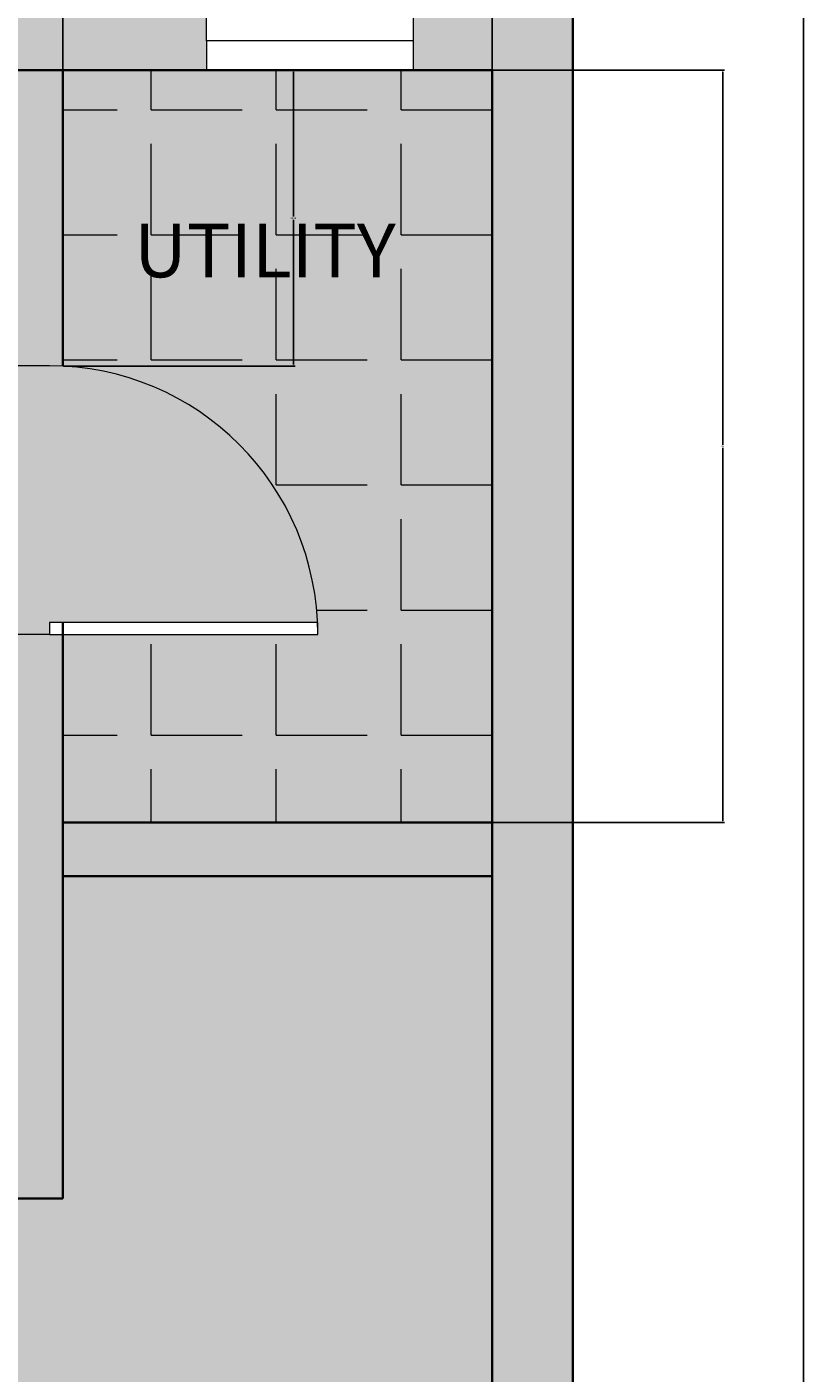
# Model space of a CAD drawing. Units: inches. Extents: x 3024 to 3952, y 1308 to 1863.
# Tile 26 of 29: x 3409 to 3496, y 1633 to 1783. Entities that reach past the tile are written whole.
import ezdxf

# ---------------------------------------------------------------- set-up
doc = ezdxf.new("R2010")
doc.units = ezdxf.units.IN
for name, color, linetype, lineweight in [('A-ANNO-DIMS', 2, 'Continuous', 18), ('A-AREA-IDEN', 7, 'Continuous', 18), ('A-DOOR', 4, 'Continuous', 18), ('A-FLOR-TILE-PATT', 7, 'Continuous', 13), ('A-GLAZ', 4, 'Continuous', 18), ('A-WALL', 7, 'Continuous', 35)]:
    doc.layers.add(name, color=color, linetype=linetype, lineweight=lineweight)
doc.layers.add('A-FLOR-PATT', color=254, linetype='Continuous', lineweight=13, true_color=0xfeeab9)
doc.layers.add('A-WALL-PATT', color=254, linetype='Continuous', lineweight=13, true_color=0xcecce6)
doc.styles.get("Standard").update_dxf_attribs({"font": 'arial.ttf'})
doc.dimstyles.get("Standard").update_dxf_attribs({"dimtxt": 0.18, "dimasz": 0.18, "dimexe": 0.18, "dimexo": 0.0625, "dimgap": 0.09, "dimtad": 0, "dimtih": 1, "dimtoh": 1, "dimdec": 4, "dimzin": 0, "dimdsep": 46, "dimtxsty": 'Standard', "dimcen": 0.09, "dimadec": 0, "dimazin": 0, "dimtfac": 1, "dimtdec": 4, "dimtofl": 0, "dimtmove": 0, "dimatfit": 3, "dimfxl": 1, "dimtolj": 1, "dimtzin": 0, "dimarcsym": 0})
pattern_1 = [(0, (0, 0), (0, 13.97), [10.16, -3.81]), (90, (0, 0), (-13.97, 9e-16), [10.16, -3.81])]

# ---------------------------------------------------------------- blocks, each defined once
blk = doc.blocks.new('*U3')
for p, q in [((0, 0), (0, 6)), ((40, 0), (40, 6))]:
    blk.add_line(p, q)
blk.add_lwpolyline([(0, 0), (0, -40), (1.75, -40), (1.75, 0)], close=True)
blk.add_arc((0, 0), 40, 270, 0)
blk = doc.blocks.new('*D37')
at = {"layer": 'A-ANNO-DIMS', "color": 0, "lineweight": -2, "transparency": 16777216}
for p, q in [((3469.83, 1787.61), (3495.72, 1787.61)), ((3495.54, 1787.43), (3495.54, 1567.91)), ((3495.54, 1348.03), (3495.54, 1567.54)), ((3469.83, 1347.85), (3495.72, 1347.85))]:
    blk.add_line(p, q, dxfattribs=at)
at = {"layer": 'A-ANNO-DIMS', "color": 0, "transparency": 16777216}
for points in [[(3495.51, 1787.43), (3495.57, 1787.43), (3495.54, 1787.61)], [(3495.51, 1348.03), (3495.57, 1348.03), (3495.54, 1347.85)]]:
    blk.add_solid(points, dxfattribs=at)
at = {"layer": 'Defpoints', "color": 0, "transparency": 16777216}
for p in [(3469.76, 1787.61), (3495.54, 1787.61), (3469.76, 1347.85)]:
    blk.add_point(p, dxfattribs=at)
at = {"layer": 'A-ANNO-DIMS', "color": 0, "transparency": 16777216, "insert": (3495.54, 1567.73), "char_height": 0.18, "attachment_point": 5}
blk.add_mtext('\\A1;439.8', dxfattribs=at)
blk = doc.blocks.new('*D41')
at = {"layer": 'A-ANNO-DIMS', "color": 0, "lineweight": -2, "transparency": 16777216}
for p, q in [((3412.76, 1778.67), (3412.76, 1862.78)), ((3412.94, 1862.6), (3436.54, 1862.6)), ((3460.58, 1862.6), (3436.99, 1862.6)), ((3460.76, 1778.67), (3460.76, 1862.78))]:
    blk.add_line(p, q, dxfattribs=at)
at = {"layer": 'A-ANNO-DIMS', "color": 0, "transparency": 16777216}
for points in [[(3412.94, 1862.63), (3412.94, 1862.57), (3412.76, 1862.6)], [(3460.58, 1862.63), (3460.58, 1862.57), (3460.76, 1862.6)]]:
    blk.add_solid(points, dxfattribs=at)
at = {"layer": 'Defpoints', "color": 0, "transparency": 16777216}
for p in [(3460.76, 1862.6), (3412.76, 1778.61), (3460.76, 1778.61)]:
    blk.add_point(p, dxfattribs=at)
at = {"layer": 'A-ANNO-DIMS', "color": 0, "transparency": 16777216, "insert": (3436.76, 1862.6), "char_height": 0.18, "attachment_point": 5}
blk.add_mtext('\\A1;48', dxfattribs=at)
blk = doc.blocks.new('*D50')
at = {"layer": 'A-ANNO-DIMS', "color": 0, "lineweight": -2, "transparency": 16777216}
for p, q in [((3460.83, 1778.61), (3486.72, 1778.61)), ((3486.54, 1778.43), (3486.54, 1736.79)), ((3486.54, 1694.79), (3486.54, 1736.42)), ((3460.83, 1694.61), (3486.72, 1694.61))]:
    blk.add_line(p, q, dxfattribs=at)
at = {"layer": 'A-ANNO-DIMS', "color": 0, "transparency": 16777216}
for points in [[(3486.51, 1778.43), (3486.57, 1778.43), (3486.54, 1778.61)], [(3486.51, 1694.79), (3486.57, 1694.79), (3486.54, 1694.61)]]:
    blk.add_solid(points, dxfattribs=at)
at = {"layer": 'Defpoints', "color": 0, "transparency": 16777216}
for p in [(3460.76, 1778.61), (3460.76, 1694.61), (3486.54, 1694.61)]:
    blk.add_point(p, dxfattribs=at)
at = {"layer": 'A-ANNO-DIMS', "color": 0, "transparency": 16777216, "insert": (3486.54, 1736.61), "char_height": 0.18, "attachment_point": 5}
blk.add_mtext('\\A1;84', dxfattribs=at)
blk = doc.blocks.new('*D61')
at = {"layer": 'A-ANNO-DIMS', "color": 0, "lineweight": -2, "transparency": 16777216}
for p, q in [((3412.83, 1778.61), (3438.72, 1778.61)), ((3438.54, 1778.43), (3438.54, 1762.27)), ((3438.54, 1745.75), (3438.54, 1761.91)), ((3412.83, 1745.57), (3438.72, 1745.57))]:
    blk.add_line(p, q, dxfattribs=at)
at = {"layer": 'A-ANNO-DIMS', "color": 0, "transparency": 16777216}
for points in [[(3438.51, 1778.43), (3438.57, 1778.43), (3438.54, 1778.61)], [(3438.51, 1745.75), (3438.57, 1745.75), (3438.54, 1745.57)]]:
    blk.add_solid(points, dxfattribs=at)
at = {"layer": 'Defpoints', "color": 0, "transparency": 16777216}
for p in [(3412.76, 1778.61), (3412.76, 1745.57), (3438.54, 1745.57)]:
    blk.add_point(p, dxfattribs=at)
at = {"layer": 'A-ANNO-DIMS', "color": 0, "transparency": 16777216, "insert": (3438.54, 1762.09), "char_height": 0.18, "attachment_point": 5}
blk.add_mtext('\\A1;33.04', dxfattribs=at)

msp = doc.modelspace()

# ---------------------------------------------------------------- hatches: boundary and pattern name
at = {"layer": 'A-FLOR-PATT', "transparency": 33554531}
h = msp.add_hatch(color=256, dxfattribs=at)
h.dxf.hatch_style = 1
h.paths.add_polyline_path([(3166.764, 1628.6064), (3106.764, 1628.6064), (3106.764, 1532.6064), (3133.066, 1532.6064, -0.38700389), (3161.716, 1561.0777), (3161.716, 1561.1064), (3163.0285, 1561.1064), (3163.0285, 1532.6064), (3166.764, 1532.6064)])
h.paths.add_polyline_path([(3123.904, 1600.7821), (3117.9039, 1602.7821), (3117.9039, 1599.7821), (3119.4039, 1599.7821), (3119.4039, 1596.7821), (3118.4039, 1596.7821), (3118.4039, 1598.7821), (3117.9039, 1598.7821), (3117.9039, 1596.2821), (3109.9039, 1596.2821), (3109.9039, 1617.2821), (3117.9039, 1617.2821), (3117.9039, 1610.7821), (3123.9038, 1612.7821, -0.70257121), (3137.9039, 1606.7822, -0.70256205)], flags=16)
h.paths.add_polyline_path([(3123.9039, 1602.7822), (3123.9039, 1610.7822, -0.73453329), (3136.9039, 1606.7822, -0.73452973)], flags=0)
h.paths.add_polyline_path([(3116.1539, 1597.2821), (3111.9039, 1597.2821, -0.41421356), (3110.9039, 1598.0321), (3110.9039, 1615.2821, -0.41421356), (3111.6539, 1616.2821), (3115.9039, 1616.2821, -0.41421356), (3116.9039, 1615.5321), (3116.9039, 1598.2821, -0.41421356)], flags=0)
h.paths.add_polyline_path([(3292.764, 1778.6064), (3232.764, 1778.6064), (3232.764, 1694.6064), (3236.1584, 1694.6064), (3236.1584, 1723.1064), (3237.4709, 1723.1064), (3237.4709, 1723.0777, -0.38700389), (3266.1209, 1694.6064), (3292.764, 1694.6064)])
h.paths.add_polyline_path([(3263.6843, 1748.8282, -0.70256205), (3257.6842, 1762.8281), (3259.6842, 1768.8281), (3256.6842, 1768.8281), (3256.6842, 1767.3281), (3253.6842, 1767.3281), (3253.6842, 1768.3281), (3255.6842, 1768.3281), (3255.6842, 1768.8281), (3253.1842, 1768.8281), (3253.1842, 1776.8281), (3274.1842, 1776.8281), (3274.1842, 1768.8281), (3267.6842, 1768.8281), (3269.6842, 1762.8282, -0.70257121)], flags=16)
h.paths.add_polyline_path([(3263.6842, 1749.8282, -0.73452973), (3259.6842, 1762.8281), (3267.6843, 1762.8281, -0.73453329)], flags=0)
h.paths.add_polyline_path([(3255.1842, 1769.8281, -0.41421356), (3254.1842, 1770.5781), (3254.1842, 1774.8281, -0.41421356), (3254.9342, 1775.8281), (3272.1842, 1775.8281, -0.41421356), (3273.1842, 1775.0781), (3273.1842, 1770.8281, -0.41421356), (3272.4342, 1769.8281)], flags=0)
h.paths.add_polyline_path([(3460.764, 1778.6064), (3412.764, 1778.6064), (3412.764, 1745.5689, -0.38700389), (3441.2353, 1716.9189), (3441.264, 1716.9189), (3441.264, 1715.6064), (3412.764, 1715.6064), (3412.764, 1694.6064), (3460.764, 1694.6064)])
h.paths.add_polyline_path([(3121.3033, 1577.378), (3153.693, 1577.378), (3153.693, 1586.6752), (3121.3033, 1586.6752)], flags=24)
h.paths.add_polyline_path([(3245.8895, 1726.2997), (3278.2793, 1726.2997), (3278.2793, 1735.5968), (3245.8895, 1735.5968)], flags=24)
h.paths.add_polyline_path([(3419.204, 1753.8578), (3453.3997, 1753.8578), (3453.3997, 1762.9956), (3419.204, 1762.9956)], flags=24)
at = {"layer": 'A-FLOR-PATT', "transparency": 33554528}
h = msp.add_hatch(color=256, dxfattribs=at)
h.dxf.hatch_style = 1
h.paths.add_polyline_path([(3460.764, 1688.6064), (3412.764, 1688.6064), (3412.764, 1694.6064), (3460.764, 1694.6064), (3460.764, 1778.6064), (3406.764, 1778.6064), (3406.764, 1759.9514), (3318.2981, 1759.9514), (3318.2981, 1658.6064), (3322.5356, 1658.6064), (3322.5356, 1652.6064), (3292.764, 1652.6064), (3292.764, 1778.6064), (3106.764, 1778.6064), (3106.764, 1628.6064), (3172.764, 1628.6064), (3172.764, 1532.6064), (3166.764, 1532.6064), (3166.764, 1628.6064), (3106.764, 1628.6064), (3106.764, 1356.8452), (3202.812, 1356.8452), (3202.812, 1354.2534), (3202.812, 1353.8388), (3202.812, 1351.1212), (3202.812, 1347.8452), (3277.764, 1347.8452), (3277.764, 1353.8452), (3277.764, 1356.8452), (3277.764, 1442.6064), (3460.764, 1442.6064)])
h.paths.add_polyline_path([(3216.238, 1527.2064), (3216.238, 1491.2064), (3214.663, 1491.2064), (3214.663, 1491.2409, -0.39662236), (3180.243, 1526.6064), (3163.0285, 1526.6064), (3163.0285, 1531.1064), (3161.716, 1531.1064), (3161.716, 1561.1064), (3163.0285, 1561.1064), (3163.0285, 1531.1064), (3163.0285, 1526.6064), (3180.243, 1526.6064, 0.39662236), (3214.663, 1491.2409), (3214.663, 1527.2064)], flags=16)
h.paths.add_polyline_path([(3227.364, 1649.8972), (3191.364, 1649.8972), (3191.364, 1651.4722), (3227.364, 1651.4722)], flags=16)
h.paths.add_polyline_path([(3323.1172, 1606.7362), (3323.8545, 1606.8514), (3323.8545, 1594.8241), (3323.1172, 1594.9393)], flags=16)
h.paths.add_polyline_path([(3324.2232, 1606.909), (3330.1216, 1607.8307), (3330.1216, 1614.1093), (3339.3495, 1614.1093), (3340.2711, 1620.0078), (3352.4136, 1620.0078), (3353.3353, 1614.1093), (3359.9941, 1614.1093), (3360.9157, 1620.0078), (3373.0582, 1620.0078), (3373.9799, 1614.1093), (3383.2077, 1614.1093), (3383.2077, 1607.8307), (3389.1062, 1606.909), (3389.1062, 1594.7665), (3383.2077, 1593.8449), (3383.2077, 1587.5663), (3373.9799, 1587.5663), (3373.0583, 1581.6678), (3360.9157, 1581.6678), (3359.9941, 1587.5663), (3353.3353, 1587.5663), (3352.4136, 1581.6678), (3340.2711, 1581.6678), (3339.3495, 1587.5663), (3330.1216, 1587.5663), (3330.1216, 1593.8449), (3324.2232, 1594.7665)], flags=16)
h.paths.add_polyline_path([(3236.1584, 1693.1064), (3236.1584, 1723.1064), (3237.4709, 1723.1064), (3237.4709, 1693.1064)], flags=16)
h.paths.add_polyline_path([(3373.2158, 1600.6847), (3373.7965, 1600.7303), (3374.3268, 1600.7874), (3374.8132, 1600.8531), (3375.2621, 1600.9247), (3375.6801, 1600.9991), (3376.0736, 1601.0735), (3376.6855, 1601.19), (3377.366, 1601.3023), (3378.0667, 1601.3814), (3378.8026, 1601.4123), (3379.5865, 1601.3839), (3380.4537, 1601.2948), (3381.301, 1601.1717), (3382.0317, 1601.0433), (3382.4398, 1600.9607), (3382.6252, 1600.9201), (3382.919, 1600.8507), (3382.9044, 1600.8531), (3382.842, 1600.8678), (3382.7541, 1600.8896), (3382.6252, 1600.9201), (3382.4398, 1600.9607), (3382.1868, 1601.0119), (3381.8738, 1601.0711), (3381.5125, 1601.1346), (3381.1149, 1601.1988), (3380.6928, 1601.2601), (3380.2581, 1601.3149), (3379.8226, 1601.3597), (3379.3984, 1601.3908), (3378.9944, 1601.4054), (3378.6092, 1601.4042), (3378.2384, 1601.3886), (3377.8777, 1601.36), (3377.5227, 1601.32), (3377.1691, 1601.2698), (3376.8127, 1601.211), (3376.4491, 1601.145), (3376.0736, 1601.0735), (3375.4177, 1600.9494), (3374.5542, 1600.8119), (3373.5044, 1600.6988)], flags=0)
h.paths.add_polyline_path([(3380.0253, 1596.7351), (3380.499, 1596.6659), (3380.9706, 1596.6119), (3381.4375, 1596.5791), (3381.8971, 1596.5736), (3382.5886, 1596.6167), (3382.7848, 1596.6692), (3382.1465, 1596.5706), (3381.236, 1596.5815), (3380.3199, 1596.6865)], flags=0)
h.paths.add_polyline_path([(3369.6414, 1603.9617), (3370.1589, 1604.0021), (3370.6218, 1604.0539), (3371.0335, 1604.1173), (3371.3978, 1604.1921), (3371.7181, 1604.2785), (3371.9984, 1604.3761), (3372.2441, 1604.483), (3372.4611, 1604.5972), (3372.655, 1604.7163), (3372.8317, 1604.8384), (3372.9968, 1604.9611), (3373.3703, 1605.2455), (3373.8426, 1605.5328), (3374.4624, 1605.7539), (3375.1058, 1605.8302), (3375.7221, 1605.8261), (3376.4109, 1605.76), (3377.1534, 1605.6376), (3377.8945, 1605.473), (3378.1382, 1605.409), (3377.7394, 1605.5074), (3377.3509, 1605.5937), (3376.9704, 1605.6677), (3376.5999, 1605.7288), (3376.2417, 1605.7762), (3375.8979, 1605.8092), (3375.5707, 1605.8271), (3375.2621, 1605.8291), (3374.9745, 1605.8146), (3374.7092, 1605.7832), (3374.4647, 1605.7359), (3374.239, 1605.6742), (3374.0298, 1605.5996), (3373.835, 1605.5134), (3373.6525, 1605.4171), (3373.4801, 1605.3123), (3373.3156, 1605.2002), (3373.1562, 1605.0825), (3372.7603, 1604.781), (3372.236, 1604.4588), (3371.5738, 1604.2283), (3370.8493, 1604.0794), (3369.9262, 1603.976)], flags=0)
h.paths.add_polyline_path([(3366.7533, 1606.5832), (3367.1713, 1606.5519), (3367.5378, 1606.5374), (3367.8568, 1606.5394), (3368.1325, 1606.5573), (3368.3694, 1606.5903), (3368.5717, 1606.6377), (3368.7438, 1606.6988), (3368.89, 1606.7728), (3369.0146, 1606.8591), (3369.121, 1606.9568), (3369.2094, 1607.0646), (3369.2792, 1607.181), (3369.3295, 1607.3046), (3369.3596, 1607.4339), (3369.3688, 1607.5676), (3369.3565, 1607.7042), (3369.3218, 1607.8422), (3369.2649, 1607.9804), (3369.1893, 1608.1187), (3369.0993, 1608.2569), (3368.9992, 1608.3952), (3368.8934, 1608.5334), (3368.7861, 1608.6717), (3368.6817, 1608.8099), (3368.4212, 1609.1804), (3368.2685, 1609.7106), (3368.4883, 1610.1814), (3369.0537, 1610.4604), (3369.6717, 1610.5097), (3370.2812, 1610.3612), (3370.4805, 1610.2968), (3370.1882, 1610.3839), (3369.9284, 1610.4472), (3369.6905, 1610.4842), (3369.4662, 1610.4933), (3369.2555, 1610.4765), (3369.0608, 1610.4367), (3368.884, 1610.3767), (3368.7274, 1610.2994), (3368.5931, 1610.2077), (3368.4833, 1610.1045), (3368.4002, 1609.9927), (3368.3451, 1609.8747), (3368.3166, 1609.7517), (3368.3127, 1609.6244), (3368.331, 1609.4935), (3368.3696, 1609.3597), (3368.4261, 1609.2237), (3368.4985, 1609.0863), (3368.5845, 1608.9482), (3368.6817, 1608.8099), (3368.7861, 1608.6717), (3368.8934, 1608.5334), (3368.9992, 1608.3952), (3369.0993, 1608.2569), (3369.3398, 1607.8876), (3369.3941, 1607.2896), (3368.9774, 1606.7817), (3368.3928, 1606.5742), (3367.7162, 1606.5303), (3367.0044, 1606.5585)], flags=0)
h.paths.add_polyline_path([(3362.1859, 1610.2589), (3362.5478, 1610.2845), (3362.8348, 1610.3275), (3363.0585, 1610.3863), (3363.2303, 1610.4595), (3363.3619, 1610.5457), (3363.463, 1610.6432), (3363.5376, 1610.7502), (3363.5876, 1610.8643), (3363.6153, 1610.9834), (3363.6229, 1611.1055), (3363.6125, 1611.2283), (3363.5861, 1611.3496), (3363.5462, 1611.4673), (3363.4949, 1611.5797), (3363.4358, 1611.6871), (3363.3723, 1611.7902), (3363.3081, 1611.8897), (3363.2468, 1611.9863), (3363.192, 1612.0808), (3363.0258, 1612.4261), (3363.3371, 1612.8672), (3363.9008, 1612.9782), (3364.4822, 1612.9641), (3365.1098, 1612.9074), (3365.328, 1612.8805), (3364.9615, 1612.9208), (3364.6426, 1612.9496), (3364.3668, 1612.9669), (3364.1299, 1612.9726), (3363.9276, 1612.9669), (3363.7555, 1612.9496), (3363.6093, 1612.9208), (3363.4848, 1612.8805), (3363.3782, 1612.8289), (3363.2889, 1612.7672), (3363.2169, 1612.6969), (3363.1622, 1612.6193), (3363.1247, 1612.5361), (3363.1046, 1612.4484), (3363.1017, 1612.358), (3363.1161, 1612.266), (3363.1472, 1612.1738), (3363.192, 1612.0808), (3363.2468, 1611.9863), (3363.3081, 1611.8897), (3363.3723, 1611.7902), (3363.4358, 1611.6871), (3363.6363, 1611.323), (3363.5979, 1610.7003), (3363.0863, 1610.3651), (3362.3983, 1610.2622)], flags=0)
h.paths.add_polyline_path([(3352.356, 1581.2991), (3352.2408, 1580.5618), (3340.4439, 1580.5618), (3340.3287, 1581.2991)], flags=16)
h.paths.add_polyline_path([(3340.4439, 1621.1137), (3352.2408, 1621.1137), (3352.356, 1620.3764), (3340.3287, 1620.3764)], flags=16)
h.paths.add_polyline_path([(3278.4282, 1504.7424), (3290.3831, 1504.7424), (3290.3831, 1502.7499), (3291.0473, 1502.7499), (3291.0473, 1494.7799), (3290.3831, 1494.7799), (3290.3831, 1494.1158), (3291.0473, 1494.1158), (3291.0473, 1486.1458), (3290.3831, 1486.1458), (3290.3831, 1484.1533), (3291.0473, 1484.1533), (3291.0473, 1483.4892, -0.09090909), (3291.0473, 1468.8776), (3291.0473, 1468.2135), (3290.3831, 1468.2135), (3290.3831, 1464.8926), (3278.4282, 1464.8926), (3278.4282, 1472.8626), (3277.764, 1473.5268), (3277.764, 1478.84), (3278.4282, 1479.5042)], flags=16)
h.paths.add_polyline_path([(3278.7603, 1504.4103), (3290.051, 1504.4103), (3290.051, 1465.2247), (3278.7603, 1465.2247)], flags=0)
h.paths.add_polyline_path([(3123.904, 1600.7821), (3117.9039, 1602.7821), (3117.9039, 1599.7821), (3119.4039, 1599.7821), (3119.4039, 1596.7821), (3118.4039, 1596.7821), (3118.4039, 1598.7821), (3117.9039, 1598.7821), (3117.9039, 1596.2821), (3109.9039, 1596.2821), (3109.9039, 1617.2821), (3117.9039, 1617.2821), (3117.9039, 1610.7821), (3123.9038, 1612.7821, -0.70257121), (3137.9039, 1606.7822, -0.70256205)], flags=16)
h.paths.add_polyline_path([(3123.9039, 1602.7822), (3123.9039, 1610.7822, -0.73453329), (3136.9039, 1606.7822, -0.73452973)], flags=0)
h.paths.add_polyline_path([(3177.972, 1689.6473), (3109.2405, 1689.6473), (3109.2405, 1741.1959), (3177.972, 1741.1959)], flags=16)
h.paths.add_polyline_path([(3373.0006, 1581.2991), (3372.8854, 1580.5618), (3361.0885, 1580.5618), (3360.9733, 1581.2991)], flags=16)
h.paths.add_polyline_path([(3361.0885, 1621.1137), (3372.8854, 1621.1137), (3373.0006, 1620.3764), (3360.9733, 1620.3764)], flags=16)
h.paths.add_polyline_path([(3116.9039, 1598.2821, -0.41421356), (3116.1539, 1597.2821), (3111.9039, 1597.2821, -0.41421356), (3110.9039, 1598.0321), (3110.9039, 1615.2821, -0.41421356), (3111.6539, 1616.2821), (3115.9039, 1616.2821, -0.41421356), (3116.9039, 1615.5321)], flags=0)
h.paths.add_polyline_path([(3121.6122, 1728.1369), (3121.6122, 1696.5205), (3110.2715, 1696.5205), (3110.2715, 1714.3906), (3121.6122, 1714.3906), (3121.6122, 1716.4526), (3110.2715, 1716.4526), (3110.2715, 1734.3228), (3123.3304, 1734.3228), (3123.3304, 1729.8552), (3134.6711, 1741.1959), (3134.6711, 1728.1369)], flags=0)
h.paths.add_polyline_path([(3389.4748, 1606.8514), (3390.2122, 1606.7362), (3390.2122, 1594.9393), (3389.4748, 1594.8241)], flags=16)
h.paths.add_polyline_path([(3257.6842, 1762.8281), (3259.6842, 1768.8281), (3256.6842, 1768.8281), (3256.6842, 1767.3281), (3253.6842, 1767.3281), (3253.6842, 1768.3281), (3255.6842, 1768.3281), (3255.6842, 1768.8281), (3253.1842, 1768.8281), (3253.1842, 1776.8281), (3274.1842, 1776.8281), (3274.1842, 1768.8281), (3267.6842, 1768.8281), (3269.6842, 1762.8282, -0.70257121), (3263.6843, 1748.8282, -0.70256205)], flags=16)
h.paths.add_polyline_path([(3259.6842, 1762.8281), (3267.6843, 1762.8281, -0.73453329), (3263.6842, 1749.8282, -0.73452973)], flags=0)
h.paths.add_polyline_path([(3411.264, 1715.6064), (3411.264, 1716.9189), (3441.264, 1716.9189), (3441.264, 1715.6064)], flags=16)
h.paths.add_polyline_path([(3178.3806, 1449.1876), (3178.3806, 1397.639), (3109.6491, 1397.639), (3109.6491, 1449.1876)], flags=16)
h.paths.add_polyline_path([(3397.1501, 1541.7146), (3419.6183, 1541.7146), (3419.6183, 1496.7783), (3397.1501, 1496.7783)], flags=16)
h.paths.add_polyline_path([(3254.1842, 1770.5781), (3254.1842, 1774.8281, -0.41421356), (3254.9342, 1775.8281), (3272.1842, 1775.8281, -0.41421356), (3273.1842, 1775.0781), (3273.1842, 1770.8281, -0.41421356), (3272.4342, 1769.8281), (3255.1842, 1769.8281, -0.41421356)], flags=0)
h.paths.add_polyline_path([(3403.672, 1500.7601), (3403.6016, 1500.3997), (3403.5328, 1500.0441), (3403.4662, 1499.6867), (3403.4027, 1499.3226), (3403.3464, 1498.9532), (3403.3025, 1498.5811), (3403.2759, 1498.2091), (3403.2714, 1497.8401), (3403.3064, 1497.2813), (3403.3491, 1497.1219), (3403.2689, 1497.6395), (3403.2778, 1498.3719), (3403.3635, 1499.0984), (3403.4889, 1499.8168), (3403.6016, 1500.3997), (3403.672, 1500.7601), (3403.744, 1501.1315), (3403.817, 1501.5205), (3403.891, 1501.9336), (3403.9656, 1502.3769), (3404.0404, 1502.8572), (3404.115, 1503.3786), (3404.2264, 1504.2311), (3404.2571, 1504.5223), (3404.1552, 1503.6598), (3404.0063, 1502.6193), (3403.8604, 1501.7518), (3403.744, 1501.1315)], flags=0)
h.paths.add_polyline_path([(3406.5868, 1505.0416), (3406.6121, 1504.5236), (3406.6492, 1504.0526), (3406.6956, 1503.624), (3406.7491, 1503.2333), (3406.8072, 1502.8759), (3406.8676, 1502.5473), (3406.9281, 1502.243), (3407.0268, 1501.7597), (3407.1416, 1501.1368), (3407.2087, 1500.3904), (3407.1804, 1499.6703), (3407.1078, 1498.9956), (3407.0074, 1498.3199), (3406.8809, 1497.6059), (3406.7403, 1496.9627), (3406.7418, 1496.9824), (3406.7491, 1497.0249), (3406.8229, 1497.3409), (3406.8364, 1497.4025), (3406.878, 1497.6078), (3406.9261, 1497.8614), (3406.9777, 1498.1526), (3407.0298, 1498.4712), (3407.0797, 1498.8068), (3407.1243, 1499.149), (3407.1607, 1499.4874), (3407.1859, 1499.8115), (3407.1978, 1500.1137), (3407.1969, 1500.3962), (3407.1841, 1500.6642), (3407.1609, 1500.9225), (3407.1284, 1501.1761), (3407.0876, 1501.43), (3407.0398, 1501.6891), (3406.9862, 1501.9585), (3406.8832, 1502.4628), (3406.7712, 1503.0713), (3406.6657, 1503.8424), (3406.5924, 1504.7735)], flags=0)
h.paths.add_polyline_path([(3409.2517, 1507.8962), (3409.2752, 1507.4282), (3409.3079, 1507.0076), (3409.3501, 1506.6314), (3409.4015, 1506.2969), (3409.4624, 1506.0009), (3409.5326, 1505.7406), (3409.6119, 1505.5128), (3409.6988, 1505.3131), (3409.7915, 1505.1368), (3409.8883, 1504.9792), (3409.9875, 1504.8356), (3410.0872, 1504.7015), (3410.1859, 1504.572), (3410.4508, 1504.2132), (3410.7205, 1503.6035), (3410.8059, 1502.8824), (3410.7619, 1502.0875), (3410.6122, 1501.2299), (3410.4402, 1500.6169), (3410.2538, 1500.0031), (3410.0536, 1499.3219), (3409.9909, 1499.0812), (3410.1761, 1499.7472), (3410.3596, 1500.3513), (3410.4512, 1500.6561), (3410.5312, 1500.9412), (3410.6013, 1501.226), (3410.6614, 1501.512), (3410.7111, 1501.7964), (3410.7496, 1502.0763), (3410.7764, 1502.3489), (3410.7909, 1502.6114), (3410.7926, 1502.8608), (3410.7808, 1503.0944), (3410.7553, 1503.31), (3410.7169, 1503.5087), (3410.6667, 1503.6921), (3410.6061, 1503.8621), (3410.5361, 1504.0203), (3410.4578, 1504.1686), (3410.3726, 1504.3088), (3410.2815, 1504.4424), (3410.1859, 1504.572), (3410.0872, 1504.7015), (3409.859, 1505.0083), (3409.5943, 1505.5117), (3409.4266, 1506.1336), (3409.324, 1506.8011), (3409.2586, 1507.6407)], flags=0)
h.paths.add_polyline_path([(3411.4914, 1510.5878), (3411.4432, 1510.1586), (3411.4054, 1509.775), (3411.38, 1509.4354), (3411.3681, 1509.1376), (3411.3698, 1508.8784), (3411.3843, 1508.6542), (3411.4112, 1508.4618), (3411.4497, 1508.2974), (3411.4994, 1508.1575), (3411.5595, 1508.0388), (3411.6296, 1507.9375), (3411.7097, 1507.851), (3411.802, 1507.7792), (3411.9096, 1507.7225), (3412.0353, 1507.6817), (3412.1821, 1507.6572), (3412.3528, 1507.6496), (3412.5505, 1507.6597), (3412.778, 1507.6879), (3413.0364, 1507.7341), (3413.3194, 1507.7955), (3413.6188, 1507.8687), (3413.9264, 1507.95), (3414.234, 1508.036), (3414.5333, 1508.1232), (3414.8163, 1508.208), (3415.0747, 1508.287), (3415.3023, 1508.3569), (3415.5007, 1508.4158), (3415.6733, 1508.4617), (3416.1158, 1508.5538), (3416.512, 1508.2591), (3416.716, 1507.6581), (3416.61, 1507.0003), (3416.3052, 1506.3411), (3415.8928, 1505.618), (3415.7339, 1505.3633), (3415.9914, 1505.791), (3416.201, 1506.1583), (3416.3666, 1506.4739), (3416.4925, 1506.7462), (3416.5828, 1506.9838), (3416.6413, 1507.1949), (3416.6725, 1507.3883), (3416.6799, 1507.5705), (3416.6662, 1507.7417), (3416.6339, 1507.9), (3416.5851, 1508.0436), (3416.5223, 1508.1709), (3416.4478, 1508.28), (3416.3639, 1508.3692), (3416.273, 1508.4368), (3416.1765, 1508.4815), (3416.0718, 1508.5047), (3415.9553, 1508.5079), (3415.8237, 1508.493), (3415.6733, 1508.4617), (3415.5007, 1508.4158), (3415.3327, 1508.3659), (3414.6495, 1508.157), (3414.0606, 1507.9855), (3413.4456, 1507.8229), (3412.8838, 1507.701), (3412.5505, 1507.6597), (3412.0748, 1507.6354), (3411.595, 1507.8883), (3411.398, 1508.4429), (3411.3624, 1508.9927), (3411.3854, 1509.5711), (3411.4578, 1510.3071)], flags=0)
h.paths.add_polyline_path([(3135.0797, 1449.1876), (3135.0797, 1436.1286), (3122.0208, 1436.1286), (3122.0208, 1404.5122), (3110.6801, 1404.5122), (3110.6801, 1422.3823), (3122.0208, 1422.3823), (3122.0208, 1424.4443), (3110.6801, 1424.4443), (3110.6801, 1442.3145), (3123.739, 1442.3145), (3123.739, 1437.8469)], flags=0)
h.paths.add_polyline_path([(3416.4944, 1514.2949), (3416.4837, 1513.8511), (3416.4893, 1513.4867), (3416.5102, 1513.1926), (3416.5451, 1512.9593), (3416.5929, 1512.7775), (3416.6524, 1512.6379), (3416.7224, 1512.531), (3416.8017, 1512.4488), (3416.8886, 1512.3882), (3416.9813, 1512.3476), (3417.0781, 1512.3251), (3417.1773, 1512.3189), (3417.277, 1512.3274), (3417.3757, 1512.3488), (3417.4713, 1512.3813), (3417.5627, 1512.4229), (3417.65, 1512.471), (3417.7338, 1512.5225), (3417.8146, 1512.5747), (3417.8931, 1512.6245), (3417.9699, 1512.6691), (3418.2968, 1512.8265), (3418.6505, 1512.4645), (3418.7037, 1511.9342), (3418.6693, 1511.3839), (3418.6076, 1510.8228), (3418.5777, 1510.5927), (3418.6197, 1510.9333), (3418.6525, 1511.2311), (3418.6759, 1511.4903), (3418.6899, 1511.7144), (3418.6946, 1511.9069), (3418.6899, 1512.0713), (3418.6759, 1512.2112), (3418.6525, 1512.33), (3418.6197, 1512.4311), (3418.5778, 1512.5177), (3418.5276, 1512.5903), (3418.4705, 1512.6488), (3418.4075, 1512.6933), (3418.3399, 1512.7237), (3418.2686, 1512.7401), (3418.1951, 1512.7424), (3418.1204, 1512.7307), (3418.0455, 1512.7055), (3417.9792, 1512.6736), (3417.65, 1512.471), (3417.5627, 1512.4229), (3417.4713, 1512.3813), (3417.3757, 1512.3488), (3417.277, 1512.3274), (3416.878, 1512.2936), (3416.5757, 1512.7549), (3416.492, 1513.3145), (3416.4808, 1514.0384)], flags=0)
h.paths.add_polyline_path([(3392.8223, 1481.9454), (3396.7707, 1481.9454), (3396.7707, 1480.9201), (3428.3585, 1480.9201), (3428.3585, 1481.9454), (3432.3069, 1481.9454), (3432.3069, 1464.8354, -0.26666697), (3392.8223, 1464.8354)], flags=16)
h.paths.add_polyline_path([(3431.203, 1547.5428), (3450.8613, 1547.5428, -0.19047621), (3450.8614, 1484.031), (3431.203, 1484.031), (3431.203, 1488.5675), (3432.3809, 1488.5675), (3432.3809, 1543.0062), (3431.203, 1543.0062)], flags=16)
h.paths.add_polyline_path([(3451.9233, 1524.86, -0.04962821), (3451.9233, 1506.7138), (3446.7921, 1506.7138), (3446.7921, 1524.86)], flags=0)
h.paths.add_polyline_path([(3460.764, 1436.6064), (3277.764, 1436.6064), (3277.764, 1356.8452), (3277.764, 1353.8452), (3460.764, 1353.8452)], flags=17)
h.paths.add_polyline_path([(3121.3033, 1577.378), (3153.693, 1577.378), (3153.693, 1586.6752), (3121.3033, 1586.6752)], flags=24)
h.paths.add_polyline_path([(3164.1457, 1464.1276), (3210.4801, 1464.1276), (3210.4801, 1473.4247), (3164.1457, 1473.4247)], flags=24)
h.paths.add_polyline_path([(3343.1909, 1505.8863), (3373.7236, 1505.8863), (3373.7236, 1515.1773), (3343.1909, 1515.1773)], flags=24)
h.paths.add_polyline_path([(3337.6353, 1564.2926), (3370.0189, 1564.2926), (3370.0189, 1573.5836), (3337.6353, 1573.5836)], flags=24)
h.paths.add_polyline_path([(3419.204, 1753.8578), (3453.3997, 1753.8578), (3453.3997, 1762.9956), (3419.204, 1762.9956)], flags=24)
h.paths.add_polyline_path([(3341.2523, 1701.0246), (3381.0761, 1701.0246), (3381.0761, 1710.3156), (3341.2523, 1710.3156)], flags=24)
h.paths.add_polyline_path([(3245.8895, 1726.2997), (3278.2793, 1726.2997), (3278.2793, 1735.5968), (3245.8895, 1735.5968)], flags=24)
h.paths.add_polyline_path([(3128.8045, 1668.6736), (3175.1389, 1668.6736), (3175.1389, 1677.9707), (3128.8045, 1677.9707)], flags=24)
h.paths.add_polyline_path([(3345.9997, 1396.0062), (3389.09, 1396.0062), (3389.09, 1405.3033), (3345.9997, 1405.3033)], flags=24)
at = {"layer": 'A-FLOR-TILE-PATT', "transparency": 33554569}
h = msp.add_hatch(dxfattribs=at)
h.set_pattern_fill('ANGLE', color=256, scale=2)
h.set_pattern_definition(pattern_1)
h.paths.add_polyline_path([(3292.764, 1778.6064), (3232.764, 1778.6064), (3232.764, 1694.6064), (3236.1584, 1694.6064), (3236.1584, 1723.1064), (3237.4709, 1723.1064), (3237.4709, 1723.0777, -0.38700389), (3266.1209, 1694.6064), (3292.764, 1694.6064)])
h.paths.add_polyline_path([(3263.6843, 1748.8282, -0.70256205), (3257.6842, 1762.8281), (3259.6842, 1768.8281), (3256.6842, 1768.8281), (3256.6842, 1767.3281), (3253.6842, 1767.3281), (3253.6842, 1768.3281), (3255.6842, 1768.3281), (3255.6842, 1768.8281), (3253.1842, 1768.8281), (3253.1842, 1776.8281), (3274.1842, 1776.8281), (3274.1842, 1768.8281), (3267.6842, 1768.8281), (3269.6842, 1762.8282, -0.70257121)], flags=16)
h.paths.add_polyline_path([(3263.6842, 1749.8282, -0.73452973), (3259.6842, 1762.8281), (3267.6843, 1762.8281, -0.73453329)], flags=0)
h.paths.add_polyline_path([(3255.1842, 1769.8281, -0.41421356), (3254.1842, 1770.5781), (3254.1842, 1774.8281, -0.41421356), (3254.9342, 1775.8281), (3272.1842, 1775.8281, -0.41421356), (3273.1842, 1775.0781), (3273.1842, 1770.8281, -0.41421356), (3272.4342, 1769.8281)], flags=0)
h.paths.add_polyline_path([(3460.764, 1436.6064), (3277.764, 1436.6064), (3277.764, 1356.8452), (3277.764, 1353.8452), (3460.764, 1353.8452)])
h.paths.add_polyline_path([(3166.764, 1628.6064), (3106.764, 1628.6064), (3106.764, 1532.6064), (3133.066, 1532.6064, -0.38700389), (3161.716, 1561.0777), (3161.716, 1561.1064), (3163.0285, 1561.1064), (3163.0285, 1532.6064), (3166.764, 1532.6064)])
h.paths.add_polyline_path([(3123.904, 1600.7821), (3117.9039, 1602.7821), (3117.9039, 1599.7821), (3119.4039, 1599.7821), (3119.4039, 1596.7821), (3118.4039, 1596.7821), (3118.4039, 1598.7821), (3117.9039, 1598.7821), (3117.9039, 1596.2821), (3109.9039, 1596.2821), (3109.9039, 1617.2821), (3117.9039, 1617.2821), (3117.9039, 1610.7821), (3123.9038, 1612.7821, -0.70257121), (3137.9039, 1606.7822, -0.70256205)], flags=16)
h.paths.add_polyline_path([(3123.9039, 1602.7822), (3123.9039, 1610.7822, -0.73453329), (3136.9039, 1606.7822, -0.73452973)], flags=0)
h.paths.add_polyline_path([(3116.1539, 1597.2821), (3111.9039, 1597.2821, -0.41421356), (3110.9039, 1598.0321), (3110.9039, 1615.2821, -0.41421356), (3111.6539, 1616.2821), (3115.9039, 1616.2821, -0.41421356), (3116.9039, 1615.5321), (3116.9039, 1598.2821, -0.41421356)], flags=0)
h.paths.add_polyline_path([(3245.8895, 1726.2997), (3278.2793, 1726.2997), (3278.2793, 1735.5968), (3245.8895, 1735.5968)], flags=24)
h.paths.add_polyline_path([(3345.9997, 1396.0062), (3389.09, 1396.0062), (3389.09, 1405.3033), (3345.9997, 1405.3033)], flags=24)
h.paths.add_polyline_path([(3121.3033, 1577.378), (3153.693, 1577.378), (3153.693, 1586.6752), (3121.3033, 1586.6752)], flags=24)
h = msp.add_hatch(dxfattribs=at)
h.set_pattern_fill('ANGLE', color=256, scale=2)
h.set_pattern_definition(pattern_1)
h.paths.add_polyline_path([(3460.764, 1778.6064), (3412.764, 1778.6064), (3412.764, 1745.5689, -0.38700389), (3441.2353, 1716.9189), (3441.264, 1716.9189), (3441.264, 1715.6064), (3412.764, 1715.6064), (3412.764, 1694.6064), (3460.764, 1694.6064)])
h.paths.add_polyline_path([(3419.204, 1753.8578), (3453.3997, 1753.8578), (3453.3997, 1762.9956), (3419.204, 1762.9956)], flags=24)
at = {"layer": 'A-WALL-PATT'}
h = msp.add_hatch(color=256, dxfattribs=at)
h.dxf.hatch_style = 1
h.paths.add_polyline_path([(3106.764, 1778.6064), (3140.5977, 1778.6064), (3140.5977, 1781.8824), (3140.5977, 1784.6), (3140.5977, 1787.6064), (3097.764, 1787.6064), (3097.764, 1590.213), (3101.04, 1590.213), (3103.7576, 1590.213), (3106.764, 1590.213)])
h.paths.add_polyline_path([(3253.5314, 1781.8824), (3253.5314, 1784.6), (3253.5314, 1787.6064), (3194.6826, 1787.6064), (3194.6826, 1785.0146), (3194.6826, 1784.6), (3194.6826, 1781.8824), (3194.6826, 1778.6064), (3253.5314, 1778.6064)])
h.paths.add_polyline_path([(3333.856, 1782.2838), (3333.856, 1784.7474), (3333.856, 1787.6064), (3272.0523, 1787.6064), (3272.0523, 1785.0146), (3272.0523, 1784.6), (3272.0523, 1781.8824), (3272.0523, 1778.6064), (3333.856, 1778.6064)])
h.paths.add_polyline_path([(3428.8344, 1784.6), (3428.8344, 1787.6064), (3378.3947, 1787.6064), (3378.3947, 1784.7474), (3378.3947, 1782.2838), (3378.3947, 1778.6064), (3428.8344, 1778.6064), (3428.8344, 1781.8824)], flags=17)
h.paths.add_polyline_path([(3469.764, 1787.6064), (3451.9386, 1787.6064), (3451.9386, 1785.0146), (3451.9386, 1784.6), (3451.9386, 1781.8824), (3451.9386, 1778.6064), (3460.764, 1778.6064), (3460.764, 1353.8452), (3277.764, 1353.8452), (3277.764, 1347.8452), (3469.764, 1347.8452), (3469.764, 1353.8452)])
h.paths.add_polyline_path([(3106.764, 1571.6922), (3104.1722, 1571.6922), (3103.7576, 1571.6922), (3101.04, 1571.6922), (3097.764, 1571.6922), (3097.764, 1347.8452), (3148.7271, 1347.8452), (3148.7271, 1351.1212), (3148.7271, 1353.8388), (3148.7271, 1356.8452), (3106.764, 1356.8452)])
h.paths.add_polyline_path([(3277.764, 1532.6064), (3262.7605, 1532.6064), (3262.7605, 1582.9359), (3256.7605, 1582.9359), (3256.7605, 1532.6064), (3244.2116, 1532.6064), (3216.238, 1532.6064), (3216.238, 1527.2064), (3216.238, 1526.6064), (3271.764, 1526.6064), (3271.764, 1356.8452), (3202.812, 1356.8452), (3202.812, 1354.2534), (3202.812, 1353.8388), (3202.812, 1351.1212), (3202.812, 1347.8452), (3277.764, 1347.8452), (3277.764, 1353.8452), (3277.764, 1356.8452)])
h.paths.add_polyline_path([(3180.238, 1532.6064), (3163.0285, 1532.6064), (3163.0285, 1531.1064), (3163.0285, 1526.6064), (3180.243, 1526.6064, -0.00416688), (3180.238, 1527.2064)])
h.paths.add_polyline_path([(3133.0285, 1531.1064, -0.01250587), (3133.066, 1532.6064), (3106.764, 1532.6064), (3106.764, 1526.6064), (3133.0285, 1526.6064)], flags=17)
h.paths.add_polyline_path([(3172.764, 1628.6064), (3166.764, 1628.6064), (3166.764, 1532.6064), (3172.764, 1532.6064)])
h.paths.add_polyline_path([(3232.764, 1649.8972), (3227.364, 1649.8972), (3226.764, 1649.8972), (3226.764, 1634.6064), (3106.764, 1634.6064), (3106.764, 1628.6064), (3232.764, 1628.6064)])
h = msp.add_hatch(color=256, dxfattribs=at)
h.dxf.hatch_style = 1
h.paths.add_polyline_path([(3232.764, 1778.6064), (3226.764, 1778.6064), (3226.764, 1685.8922, -0.00416688), (3227.364, 1685.8972), (3232.764, 1685.8972)])
h.paths.add_polyline_path([(3298.764, 1778.6064), (3292.764, 1778.6064), (3292.764, 1652.6064), (3322.5356, 1652.6064), (3322.5356, 1658.6064), (3298.764, 1658.6064)])
h.paths.add_polyline_path([(3412.764, 1715.6064), (3411.264, 1715.6064), (3406.764, 1715.6064), (3406.764, 1658.6064), (3383.3911, 1658.6064), (3383.3911, 1652.6064), (3412.764, 1652.6064)])
h.paths.add_polyline_path([(3412.764, 1778.6064), (3406.764, 1778.6064), (3406.764, 1745.6064), (3411.264, 1745.6064, -0.01250587), (3412.764, 1745.5689)])
h = msp.add_hatch(color=256, dxfattribs=at)
h.dxf.hatch_style = 1
h.paths.add_polyline_path([(3460.764, 1694.6064), (3412.764, 1694.6064), (3412.764, 1688.6064), (3460.764, 1688.6064)])

# ---------------------------------------------------------------- linework, layer by layer
at = {"layer": 'A-GLAZ'}
for p, q in [((3428.8344, 1781.8824), (3428.8344, 1778.6064)), ((3451.9386, 1782.2969), (3451.9386, 1778.6064))]:
    msp.add_line(p, q, dxfattribs=at)
msp.add_lwpolyline([(3428.8344, 1784.6), (3451.9386, 1784.6), (3451.9386, 1781.8824), (3428.8344, 1781.8824)], close=True, dxfattribs=at)
at = {"layer": 'A-WALL'}
for p, q in [((3469.764, 1347.8452), (3469.764, 1787.6064)), ((3106.764, 1778.6064), (3460.764, 1778.6064)), ((3412.764, 1745.5689), (3412.764, 1778.6064)), ((3460.764, 1353.8452), (3460.764, 1778.6064)), ((3412.764, 1652.6064), (3412.764, 1716.9189)), ((3412.764, 1694.6064), (3460.764, 1694.6064)), ((3412.764, 1688.6064), (3460.764, 1688.6064)), ((3383.3911, 1652.6064), (3412.764, 1652.6064))]:
    msp.add_line(p, q, dxfattribs=at)

# ---------------------------------------------------------------- block references
at = {"layer": 'A-DOOR', "xscale": 0.75, "yscale": 0.75, "zscale": 0.75, "rotation": 90}
msp.add_blockref('*U3', (3411.264, 1715.6064), dxfattribs=at)

# ---------------------------------------------------------------- texts
at = {"layer": 'A-AREA-IDEN'}
msp.add_text('UTILITY', height=5.98971, dxfattribs=at).set_placement((3420.727, 1755.4829))

# ---------------------------------------------------------------- dimensions: what is measured, and where the dimension line sits
at = {"layer": 'A-ANNO-DIMS'}
dim = msp.add_linear_dim(base=(3460.764, 1862.6031), p1=(3412.764, 1778.6064), p2=(3460.764, 1778.6064), dimstyle='Standard', override={"dimdec": 0, "dimlfac": 1, "dimrnd": 0, "dimzin": 0, "dimdsep": 46, "dimlunit": 2}, dxfattribs=at)
dim.commit()
dim.dimension.update_dxf_attribs({"geometry": '*D41', "text_midpoint": (3436.764, 1862.6031)})
for base, p1, p2, angle, override, picture, middle in [((3495.539, 1787.6064), (3469.764, 1347.8452), (3469.764, 1787.6064), 90, {"dimdec": 1, "dimlfac": 1, "dimrnd": 0, "dimzin": 0, "dimdsep": 46, "dimlunit": 2}, '*D37', (3495.539, 1567.7258)), ((3438.539, 1745.5689), (3412.764, 1778.6064), (3412.764, 1745.5689), 270, {"dimdec": 2, "dimlfac": 1, "dimrnd": 0, "dimzin": 0, "dimdsep": 46, "dimlunit": 2}, '*D61', (3438.539, 1762.0876)), ((3486.539, 1694.6064), (3460.764, 1778.6064), (3460.764, 1694.6064), 270, {"dimdec": 0, "dimlfac": 1, "dimrnd": 0, "dimzin": 0, "dimdsep": 46, "dimlunit": 2}, '*D50', (3486.539, 1736.6064))]:
    dim = msp.add_linear_dim(base=base, p1=p1, p2=p2, angle=angle, dimstyle='Standard', override=override, dxfattribs=at)
    dim.commit()
    dim.dimension.update_dxf_attribs({"geometry": picture, "text_midpoint": middle})

doc.saveas('drawing.dxf')
